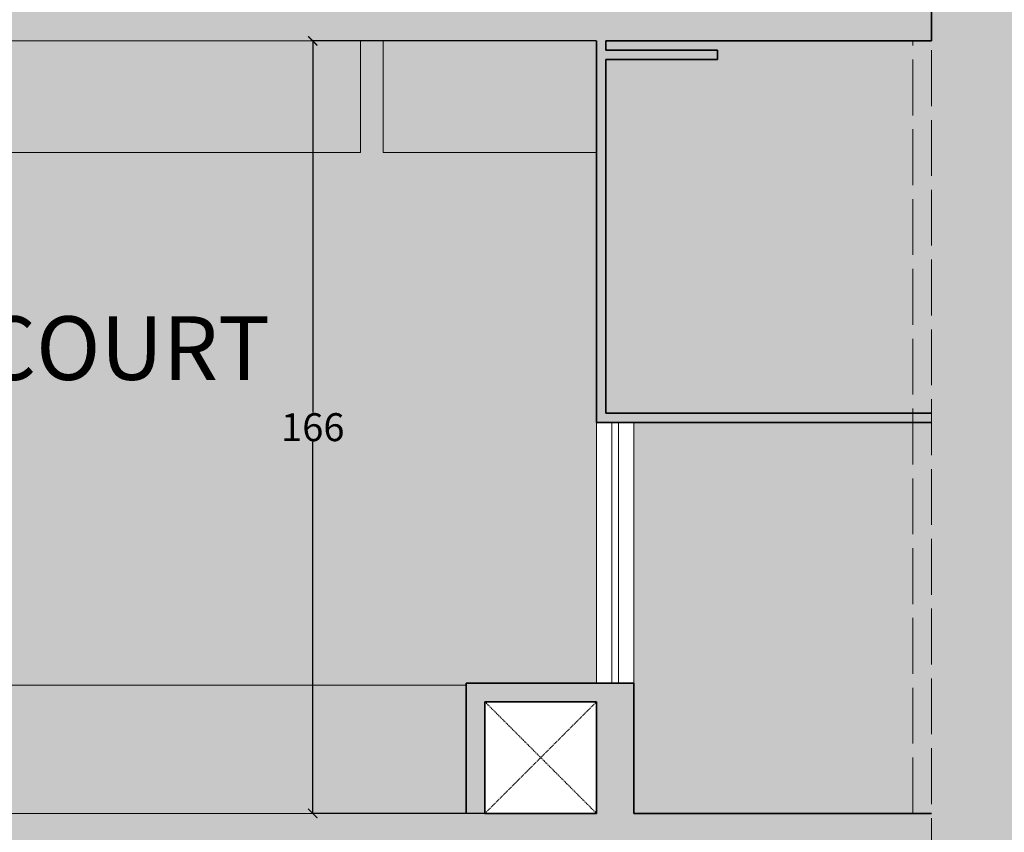
# Model space of a CAD drawing. Units: inches. Extents: x 1704 to 6393, y -157 to 1172.
# Tile 42 of 122: x 2081 to 2293, y 541 to 716. Entities that reach past the tile are written whole.
import ezdxf

# ---------------------------------------------------------------- set-up
doc = ezdxf.new("R2010")
doc.units = ezdxf.units.IN
doc.header["$MEASUREMENT"] = 0
doc.linetypes.add('ACAD_ISO02W100', pattern=[15, 12, -3])
doc.linetypes.add('HIDDEN', pattern=[0.375, 0.25, -0.125])
for name, color, linetype, lineweight in [('A-ANNO-DIMS', 7, 'Continuous', 13), ('A-AREA-IDEN', 7, 'Continuous', 18), ('A-FLOR-OPEN-HIDN', 8, 'HIDDEN', 13), ('A-WALL-OVHD', 8, 'ACAD_ISO02W100', 13), ('A-WALL-PATT', 7, 'Continuous', 13), ('GLASS PANEL FASADE', 4, 'Continuous', 18), ('L-HRDS', 8, 'Continuous', 18), ('WALLS', 7, 'Continuous', 35)]:
    doc.layers.add(name, color=color, linetype=linetype, lineweight=lineweight)
for name, color, linetype, lineweight, true_color in [('A-FLOR-PATT', 7, 'Continuous', 13, 0xf2f2f2), ('L-HRDS-PATT', 9, 'Continuous', 13, 0xc5c1ba), ('L-PLNT-PATT', 253, 'Continuous', 13, 0x9abc8f)]:
    doc.layers.add(name, color=color, linetype=linetype, lineweight=lineweight, true_color=true_color)
doc.styles.get("Standard").update_dxf_attribs({"font": 'arial.ttf'})
doc.dimstyles.get("Standard").update_dxf_attribs({"dimtxt": 6, "dimasz": 2, "dimexe": 0.18, "dimexo": 0.0625, "dimgap": 0.09, "dimtad": 0, "dimtih": 1, "dimtoh": 1, "dimdec": 1, "dimzin": 0, "dimdsep": 46, "dimlunit": 3, "dimtxsty": 'Standard', "dimblk": 'ARCHTICK', "dimcen": 0.09, "dimadec": 0, "dimazin": 0, "dimtfac": 1, "dimtdec": 1, "dimtofl": 0, "dimtmove": 0, "dimatfit": 3, "dimfxl": 1, "dimtolj": 1, "dimtzin": 0, "dimarcsym": 0})

# ---------------------------------------------------------------- blocks, each defined once
blk = doc.blocks.new('_ArchTick')
at = {"color": 0, "linetype": 'ByBlock', "const_width": 0.15}
blk.add_lwpolyline([(-0.5, -0.5), (0.5, 0.5)], dxfattribs=at)
blk = doc.blocks.new('*D93')
at = {"layer": 'A-ANNO-DIMS', "color": 0, "lineweight": -2, "transparency": 16777216}
for p, q in [((2605.29, 895.21), (1829.7, 895.21)), ((1829.88, 895.21), (1829.88, 495.87)), ((1829.88, 90.21), (1829.88, 489.56)), ((2605.29, 90.21), (1829.7, 90.21))]:
    blk.add_line(p, q, dxfattribs=at)
at = {"layer": 'Defpoints', "color": 0, "lineweight": -3, "transparency": 16777216}
for p in [(2605.35, 895.21), (1829.88, 90.21), (2605.35, 90.21)]:
    blk.add_point(p, dxfattribs=at)
at = {"layer": 'A-ANNO-DIMS', "color": 0, "lineweight": -2, "transparency": 16777216, "xscale": 2, "yscale": 2, "zscale": 2}
for p, rotation in [((1829.88, 895.21), 90), ((1829.88, 90.21), 270)]:
    blk.add_blockref('_ArchTick', p, dxfattribs=dict(at, rotation=rotation))
at = {"layer": 'A-ANNO-DIMS', "color": 0, "transparency": 16777216, "insert": (1829.88, 492.71), "char_height": 6, "attachment_point": 5}
blk.add_mtext('\\A1;805', dxfattribs=at)
blk = doc.blocks.new('*D96')
at = {"layer": 'A-ANNO-DIMS', "color": 0, "lineweight": -2, "transparency": 16777216}
for p, q in [((2205.29, 711.21), (2144.17, 711.21)), ((2144.35, 711.21), (2144.35, 631.37)), ((2144.35, 545.21), (2144.35, 625.06)), ((2205.29, 545.21), (2144.17, 545.21))]:
    blk.add_line(p, q, dxfattribs=at)
at = {"layer": 'Defpoints', "color": 0, "lineweight": -3, "transparency": 16777216}
for p in [(2144.35, 711.21), (2205.35, 711.21), (2205.35, 545.21)]:
    blk.add_point(p, dxfattribs=at)
at = {"layer": 'A-ANNO-DIMS', "color": 0, "lineweight": -2, "transparency": 16777216, "xscale": 2, "yscale": 2, "zscale": 2}
for p, rotation in [((2144.35, 711.21), 90), ((2144.35, 545.21), 270)]:
    blk.add_blockref('_ArchTick', p, dxfattribs=dict(at, rotation=rotation))
at = {"layer": 'A-ANNO-DIMS', "color": 0, "transparency": 16777216, "insert": (2144.35, 628.21), "char_height": 6, "attachment_point": 5}
blk.add_mtext('\\A1;166', dxfattribs=at)

msp = doc.modelspace()

# ---------------------------------------------------------------- hatches: boundary and pattern name
at = {"layer": 'A-FLOR-PATT', "transparency": 33554528}
h = msp.add_hatch(color=256, dxfattribs=at)
h.dxf.hatch_style = 1
h.paths.add_polyline_path([(2325.349, 863.213), (2325.349, 887.213), (2263.349, 887.213), (2167.349, 887.213), (2081.349, 887.213), (2081.349, 719.213), (2277.349, 719.213), (2277.349, 711.213), (2277.349, 372.213), (2349.349, 372.213), (2381.349, 372.213), (2381.349, 364.213), (2353.349, 364.213), (2353.349, 270.213), (2381.349, 270.213), (2381.349, 266.213), (2357.349, 266.213), (2357.349, 98.213), (2381.349, 98.213), (2385.181, 98.213), (2386.482, 98.213), (2424.215, 98.213), (2425.516, 98.213), (2429.349, 98.213), (2597.349, 98.213), (2597.349, 146.213), (2597.349, 218.213), (2597.349, 266.213), (2423.349, 266.213), (2423.349, 270.213), (2473.349, 270.213), (2473.349, 294.213), (2477.349, 294.213), (2477.349, 270.213), (2547.349, 270.213), (2547.349, 364.213), (2477.349, 364.213), (2477.349, 318.213), (2473.349, 318.213), (2473.349, 364.213), (2423.349, 364.213), (2423.349, 372.213), (2469.349, 372.213), (2469.349, 459.213), (2469.349, 538.213), (2350.349, 538.213), (2350.349, 565.713), (2358.349, 565.713), (2358.349, 545.213), (2420.349, 545.213), (2420.349, 610.213), (2358.349, 610.213), (2358.349, 589.713), (2350.349, 589.713), (2350.349, 615.213), (2425.349, 615.213), (2425.349, 607.213), (2425.349, 546.213), (2469.349, 546.213), (2514.349, 546.213), (2514.349, 607.213), (2449.349, 607.213), (2449.349, 615.213), (2451.738, 615.213), (2451.738, 659.213), (2427.738, 659.213), (2427.738, 665.213), (2367.738, 665.213), (2367.738, 667.213), (2367.738, 711.213), (2325.349, 711.213), (2325.349, 719.213), (2325.349, 755.213), (2325.349, 763.213)])
h.paths.add_polyline_path([(2233.858, 822.533, -0.187247), (2233.858, 809.14), (2231.697, 808.804, 0.0848928), (2233.131, 814.486), (2230.424, 814.486, -0.1042581), (2228.553, 808.313), (2217.751, 807.156, -0.2222222), (2217.751, 824.517), (2228.553, 823.359, -0.1042581), (2230.424, 817.186), (2233.131, 817.186, 0.0848928), (2231.697, 822.868)], flags=16)
h.paths.add_polyline_path([(2213.621, 833.197), (2213.621, 798.475), (2156.048, 798.475), (2156.048, 833.197)], flags=16)
h.paths.add_polyline_path([(2203.932, 848.099), (2205.089, 837.296, -0.2222222), (2187.728, 837.296), (2188.885, 848.099, -0.1042581), (2195.058, 849.969), (2195.058, 852.676, 0.0848928), (2189.377, 851.242), (2189.712, 853.404, -0.187247), (2203.105, 853.404), (2203.44, 851.242, 0.0848928), (2197.759, 852.676), (2197.759, 849.969, -0.1042581)], flags=16)
h.paths.add_polyline_path([(2181.941, 837.296, -0.2222222), (2164.58, 837.296), (2165.737, 848.099, -0.1042581), (2171.91, 849.969), (2171.91, 852.676, 0.0848928), (2166.229, 851.242), (2166.564, 853.404, -0.187247), (2179.957, 853.404), (2180.292, 851.242, 0.0848928), (2174.611, 852.676), (2174.611, 849.969, -0.1042581), (2180.784, 848.099)], flags=16)
h.paths.add_polyline_path([(2205.089, 794.376), (2203.932, 783.574, -0.1042581), (2197.759, 781.703), (2197.759, 778.996, 0.0848928), (2203.44, 780.43), (2203.105, 778.269, -0.187247), (2189.712, 778.269), (2189.377, 780.43, 0.0848928), (2195.058, 778.996), (2195.058, 781.703, -0.1042581), (2188.885, 783.574), (2187.728, 794.376, -0.2222222)], flags=16)
h.paths.add_polyline_path([(2181.941, 794.376), (2180.784, 783.574, -0.1042581), (2174.611, 781.703), (2174.611, 778.996, 0.0848928), (2180.292, 780.43), (2179.957, 778.269, -0.187247), (2166.564, 778.269), (2166.229, 780.43, 0.0848928), (2171.91, 778.996), (2171.91, 781.703, -0.1042581), (2165.737, 783.574), (2164.58, 794.376, -0.2222222)], flags=16)
h.paths.add_polyline_path([(2151.918, 807.156), (2141.116, 808.313, -0.1042581), (2139.245, 814.486), (2136.539, 814.486, 0.0848928), (2137.972, 808.804), (2135.811, 809.14, -0.187247), (2135.811, 822.533), (2137.972, 822.868, 0.0848928), (2136.539, 817.186), (2139.245, 817.186, -0.1042581), (2141.116, 823.359), (2151.918, 824.517, -0.2222222)], flags=16)
h.paths.add_polyline_path([(2357.868, 363.41), (2358.814, 363.41, 0.7537605)], flags=16)
h.paths.add_polyline_path([(2372.241, 363.117), (2372.248, 363.117), (2372.248, 363.343), (2371.302, 363.343), (2371.302, 363.139, -1.3603913)], flags=16)
h.paths.add_polyline_path([(2371.309, 272.716), (2371.302, 272.716), (2371.302, 272.49), (2372.248, 272.49), (2372.248, 272.693, -1.3603913)], flags=16)
h.paths.add_polyline_path([(2357.875, 272.716), (2357.868, 272.716), (2357.868, 272.49), (2358.814, 272.49), (2358.814, 272.693, -1.3603913)], flags=16)
h.paths.add_polyline_path([(2353.769, 363.074), (2376.347, 363.074), (2376.347, 272.759), (2353.769, 272.759)], flags=16)
h.paths.add_polyline_path([(2354.772, 362.07), (2375.344, 362.07), (2375.344, 273.762), (2354.772, 273.762)], flags=0)
h.paths.add_polyline_path([(2357.868, 363.343), (2358.814, 363.343), (2358.814, 363.117), (2357.868, 363.117)], flags=16)
h.paths.add_polyline_path([(2359.288, 359.184), (2359.288, 360.063), (2370.828, 360.063), (2370.828, 359.184), (2374.332, 359.184), (2374.332, 358.464), (2372.835, 358.464), (2372.835, 357.541), (2374.332, 357.541), (2374.332, 356.82), (2372.835, 356.82), (2372.835, 355.898), (2374.332, 355.898), (2374.332, 355.177), (2372.835, 355.177), (2372.835, 354.254), (2374.332, 354.254), (2374.332, 353.534), (2372.835, 353.534), (2372.835, 352.611), (2374.332, 352.611), (2374.332, 351.89), (2372.835, 351.89), (2372.835, 350.968), (2374.332, 350.968), (2374.332, 350.247), (2372.835, 350.247), (2372.835, 349.324), (2374.332, 349.324), (2374.332, 348.604), (2372.835, 348.604), (2372.835, 347.681), (2374.332, 347.681), (2374.332, 346.96), (2372.835, 346.96), (2372.835, 346.038), (2374.332, 346.038), (2374.332, 345.317), (2372.835, 345.317), (2372.835, 344.395), (2374.332, 344.395), (2374.332, 343.674), (2372.835, 343.674), (2372.835, 342.751), (2374.332, 342.751), (2374.332, 342.03), (2372.835, 342.03), (2372.835, 341.108), (2374.332, 341.108), (2374.332, 340.387), (2372.835, 340.387), (2372.835, 339.465), (2374.332, 339.465), (2374.332, 338.744), (2372.835, 338.744), (2372.835, 337.821), (2374.332, 337.821), (2374.332, 337.1), (2372.835, 337.1), (2372.835, 336.178), (2374.332, 336.178), (2374.332, 335.457), (2372.835, 335.457), (2372.835, 334.535), (2374.332, 334.535), (2374.332, 333.814), (2372.835, 333.814), (2372.835, 332.891), (2374.332, 332.891), (2374.332, 332.171), (2372.835, 332.171), (2372.835, 331.248), (2374.332, 331.248), (2374.332, 330.527), (2372.835, 330.527), (2372.835, 329.605), (2374.332, 329.605), (2374.332, 328.884), (2372.835, 328.884), (2372.835, 327.961), (2374.332, 327.961), (2374.332, 327.241), (2372.835, 327.241), (2372.835, 326.318), (2374.332, 326.318), (2374.332, 325.597), (2372.835, 325.597), (2372.835, 324.675), (2374.332, 324.675), (2374.332, 323.954), (2372.835, 323.954), (2372.835, 323.031), (2374.332, 323.031), (2374.332, 322.311), (2372.835, 322.311), (2372.835, 321.388), (2374.332, 321.388), (2374.332, 320.667), (2372.835, 320.667), (2372.835, 319.745), (2374.332, 319.745), (2374.332, 319.024), (2372.835, 319.024), (2372.835, 318.102), (2374.332, 318.102), (2374.332, 317.381), (2372.835, 317.381), (2372.835, 316.458), (2374.332, 316.458), (2374.332, 315.737), (2372.835, 315.737), (2372.835, 314.815), (2374.332, 314.815), (2374.332, 314.094), (2372.835, 314.094), (2372.835, 313.172), (2374.332, 313.172), (2374.332, 312.451), (2372.835, 312.451), (2372.835, 311.528), (2374.332, 311.528), (2374.332, 310.807), (2372.835, 310.807), (2372.835, 309.885), (2374.332, 309.885), (2374.332, 309.164), (2372.835, 309.164), (2372.835, 308.242), (2374.332, 308.242), (2374.332, 307.521), (2372.835, 307.521), (2372.835, 306.598), (2374.332, 306.598), (2374.332, 305.878), (2372.835, 305.878), (2372.835, 304.955), (2374.332, 304.955), (2374.332, 304.234), (2372.835, 304.234), (2372.835, 303.312), (2374.332, 303.312), (2374.332, 302.591), (2372.835, 302.591), (2372.835, 301.668), (2374.332, 301.668), (2374.332, 300.948), (2372.835, 300.948), (2372.835, 300.025), (2374.332, 300.025), (2374.332, 299.304), (2372.835, 299.304), (2372.835, 298.382), (2374.332, 298.382), (2374.332, 297.661), (2372.835, 297.661), (2372.835, 296.738), (2374.332, 296.738), (2374.332, 296.018), (2372.835, 296.018), (2372.835, 295.095), (2374.332, 295.095), (2374.332, 294.374), (2372.835, 294.374), (2372.835, 293.452), (2374.332, 293.452), (2374.332, 292.731), (2372.835, 292.731), (2372.835, 291.809), (2374.332, 291.809), (2374.332, 291.088), (2372.835, 291.088), (2372.835, 290.165), (2374.332, 290.165), (2374.332, 289.444), (2372.835, 289.444), (2372.835, 288.522), (2374.332, 288.522), (2374.332, 287.801), (2372.835, 287.801), (2372.835, 286.879), (2374.332, 286.879), (2374.332, 286.158), (2372.835, 286.158), (2372.835, 285.235), (2374.332, 285.235), (2374.332, 284.514), (2372.835, 284.514), (2372.835, 283.592), (2374.332, 283.592), (2374.332, 282.871), (2372.835, 282.871), (2372.835, 281.949), (2374.332, 281.949), (2374.332, 281.228), (2372.835, 281.228), (2372.835, 280.305), (2374.332, 280.305), (2374.332, 279.585), (2372.835, 279.585), (2372.835, 278.662), (2374.332, 278.662), (2374.332, 277.941), (2372.835, 277.941), (2372.835, 277.019), (2374.332, 277.019), (2374.332, 276.298), (2370.828, 276.298), (2370.828, 275.769), (2359.288, 275.769), (2359.288, 276.298), (2355.784, 276.298), (2355.784, 277.019), (2357.281, 277.019), (2357.281, 277.941), (2355.784, 277.941), (2355.784, 278.662), (2357.281, 278.662), (2357.281, 279.585), (2355.784, 279.585), (2355.784, 280.305), (2357.281, 280.305), (2357.281, 281.228), (2355.784, 281.228), (2355.784, 281.949), (2357.281, 281.949), (2357.281, 282.871), (2355.784, 282.871), (2355.784, 283.592), (2357.281, 283.592), (2357.281, 284.514), (2355.784, 284.514), (2355.784, 285.235), (2357.281, 285.235), (2357.281, 286.158), (2355.784, 286.158), (2355.784, 286.879), (2357.281, 286.879), (2357.281, 287.801), (2355.784, 287.801), (2355.784, 288.522), (2357.281, 288.522), (2357.281, 289.444), (2355.784, 289.444), (2355.784, 290.165), (2357.281, 290.165), (2357.281, 291.088), (2355.784, 291.088), (2355.784, 291.809), (2357.281, 291.809), (2357.281, 292.731), (2355.784, 292.731), (2355.784, 293.452), (2357.281, 293.452), (2357.281, 294.374), (2355.784, 294.374), (2355.784, 295.095), (2357.281, 295.095), (2357.281, 296.018), (2355.784, 296.018), (2355.784, 296.738), (2357.281, 296.738), (2357.281, 297.661), (2355.784, 297.661), (2355.784, 298.382), (2357.281, 298.382), (2357.281, 299.304), (2355.784, 299.304), (2355.784, 300.025), (2357.281, 300.025), (2357.281, 300.948), (2355.784, 300.948), (2355.784, 301.668), (2357.281, 301.668), (2357.281, 302.591), (2355.784, 302.591), (2355.784, 303.312), (2357.281, 303.312), (2357.281, 304.234), (2355.784, 304.234), (2355.784, 304.955), (2357.281, 304.955), (2357.281, 305.878), (2355.784, 305.878), (2355.784, 306.598), (2357.281, 306.598), (2357.281, 307.521), (2355.784, 307.521), (2355.784, 308.242), (2357.281, 308.242), (2357.281, 309.164), (2355.784, 309.164), (2355.784, 309.885), (2357.281, 309.885), (2357.281, 310.807), (2355.784, 310.807), (2355.784, 311.528), (2357.281, 311.528), (2357.281, 312.451), (2355.784, 312.451), (2355.784, 313.172), (2357.281, 313.172), (2357.281, 314.094), (2355.784, 314.094), (2355.784, 314.815), (2357.281, 314.815), (2357.281, 315.737), (2355.784, 315.737), (2355.784, 316.458), (2357.281, 316.458), (2357.281, 317.381), (2355.784, 317.381), (2355.784, 318.102), (2357.281, 318.102), (2357.281, 319.024), (2355.784, 319.024), (2355.784, 319.745), (2357.281, 319.745), (2357.281, 320.667), (2355.784, 320.667), (2355.784, 321.388), (2357.281, 321.388), (2357.281, 322.311), (2355.784, 322.311), (2355.784, 323.031), (2357.281, 323.031), (2357.281, 323.954), (2355.784, 323.954), (2355.784, 324.675), (2357.281, 324.675), (2357.281, 325.597), (2355.784, 325.597), (2355.784, 326.318), (2357.281, 326.318), (2357.281, 327.241), (2355.784, 327.241), (2355.784, 327.961), (2357.281, 327.961), (2357.281, 328.884), (2355.784, 328.884), (2355.784, 329.605), (2357.281, 329.605), (2357.281, 330.527), (2355.784, 330.527), (2355.784, 331.248), (2357.281, 331.248), (2357.281, 332.171), (2355.784, 332.171), (2355.784, 332.891), (2357.281, 332.891), (2357.281, 333.814), (2355.784, 333.814), (2355.784, 334.535), (2357.281, 334.535), (2357.281, 335.457), (2355.784, 335.457), (2355.784, 336.178), (2357.281, 336.178), (2357.281, 337.1), (2355.784, 337.1), (2355.784, 337.821), (2357.281, 337.821), (2357.281, 338.744), (2355.784, 338.744), (2355.784, 339.465), (2357.281, 339.465), (2357.281, 340.387), (2355.784, 340.387), (2355.784, 341.108), (2357.281, 341.108), (2357.281, 342.03), (2355.784, 342.03), (2355.784, 342.751), (2357.281, 342.751), (2357.281, 343.674), (2355.784, 343.674), (2355.784, 344.395), (2357.281, 344.395), (2357.281, 345.317), (2355.784, 345.317), (2355.784, 346.038), (2357.281, 346.038), (2357.281, 346.96), (2355.784, 346.96), (2355.784, 347.681), (2357.281, 347.681), (2357.281, 348.604), (2355.784, 348.604), (2355.784, 349.324), (2357.281, 349.324), (2357.281, 350.247), (2355.784, 350.247), (2355.784, 350.968), (2357.281, 350.968), (2357.281, 351.89), (2355.784, 351.89), (2355.784, 352.611), (2357.281, 352.611), (2357.281, 353.534), (2355.784, 353.534), (2355.784, 354.254), (2357.281, 354.254), (2357.281, 355.177), (2355.784, 355.177), (2355.784, 355.898), (2357.281, 355.898), (2357.281, 356.82), (2355.784, 356.82), (2355.784, 357.541), (2357.281, 357.541), (2357.281, 358.464), (2355.784, 358.464), (2355.784, 359.184)], flags=0)
h = msp.add_hatch(color=256, dxfattribs=at)
h.dxf.hatch_style = 1
h.paths.add_polyline_path([(2273.349, 538.213), (2081.349, 538.213), (2081.349, 372.213), (2273.349, 372.213)])
h.paths.add_polyline_path([(2189.542, 505.951), (2184.316, 505.951), (2184.316, 505.591), (2169.442, 505.591), (2169.442, 505.951), (2164.216, 505.951, -0.4142136), (2163.814, 506.353), (2163.814, 526.093, -0.4142136), (2164.216, 526.495), (2189.542, 526.495, -0.4142136), (2189.944, 526.093), (2189.944, 506.353, -0.4142136)], flags=16)
h.paths.add_polyline_path([(2200.535, 511.491), (2200.535, 526.191), (2217.621, 526.191), (2217.621, 511.491), (2214.605, 511.491, -0.3946213), (2214.203, 511.116), (2203.952, 511.116, -0.3946213), (2203.551, 511.491)], flags=16)
h.paths.add_polyline_path([(2200.736, 511.692), (2200.736, 525.99), (2203.55, 525.99), (2203.55, 523.838, 0.1045605), (2214.605, 523.838), (2214.605, 525.99), (2217.42, 525.99), (2217.42, 511.692), (2214.605, 511.692), (2214.605, 523.838, -0.1045605), (2203.55, 523.838), (2203.55, 511.692)], flags=0)
h.paths.add_polyline_path([(2203.952, 511.317, -0.4142136), (2203.751, 511.518), (2203.751, 523.591, 0.099912), (2214.404, 523.591), (2214.404, 511.518, -0.4142136), (2214.203, 511.317)], flags=0)
h.paths.add_polyline_path([(2184.084, 516.015, -0.0686795), (2169.674, 516.015), (2169.674, 522.073), (2184.084, 522.073)], flags=0)
h.paths.add_polyline_path([(2183.325, 518.606, -0.0772766), (2170.433, 518.606), (2170.433, 521.123, -0.0235462), (2183.325, 521.123)], flags=0)
h.paths.add_polyline_path([(2135.029, 507.225, -0.1405189), (2135.191, 507.834, -0.0513838), (2135.029, 507.797)], flags=16)
h.paths.add_polyline_path([(2146.318, 498.997, -0.0311848), (2144.279, 499.202, -0.1719602), (2141.865, 499.263, -0.2234326), (2139.482, 499.263, -0.1719602), (2137.068, 499.202, -0.0311848), (2135.029, 498.997, -0.066975), (2135.029, 505.313, -0.0276914), (2136.841, 505.144), (2136.841, 506.777), (2136.576, 506.777), (2136.576, 507.371, 0.039911), (2145.741, 507.448, 0.2546956), (2146.318, 507.225), (2146.318, 507.269, 0.1305786), (2146.156, 507.834, -0.0704067), (2145.953, 507.935, -0.011584), (2145.714, 508.002, -0.2546956), (2145.137, 507.779, -0.2546956), (2145.361, 508.355, -0.0259693), (2145.107, 516.407, -0.0070422), (2144.025, 516.297, -0.1828112), (2142.939, 516.218, -0.2042746), (2142.015, 516.175, -0.1805419), (2139.348, 516.174, -0.0000184), (2139.345, 516.174, -0.2035615), (2138.425, 516.217, -0.0000237), (2138.421, 516.217, -0.1818152), (2137.34, 516.296, -0.0071635), (2136.24, 516.407, 0.007166), (2136.162, 518.63, 0.314303), (2135.854, 518.974, -0.1253469), (2135.537, 518.935, -0.2546956), (2135.76, 519.512, -0.0162662), (2135.67, 519.849, -0.296972), (2135.535, 520.8, -0.227702), (2135.464, 521.698, 0.1283977), (2132.757, 521.718), (2132.757, 525.785, -0.4142136), (2133.331, 526.359), (2148.015, 526.359, -0.4142136), (2148.589, 525.785), (2148.589, 521.718, -0.0118936), (2148.835, 521.65, -0.2546956), (2149.412, 521.873, -0.2546956), (2149.188, 521.296, -0.0417628), (2149.188, 508.355, -0.2546956), (2149.412, 507.779, -0.2546956), (2148.835, 508.002, -0.011584), (2148.596, 507.935, -0.2124435), (2147.949, 507.813, -0.2363999), (2147.423, 507.772, -0.3143526), (2147.126, 507.772, -0.2363999), (2146.6, 507.813, -0.0879275), (2146.318, 507.797), (2146.318, 507.225, -0.2546956), (2145.741, 507.448, -0.0042329), (2144.771, 507.371), (2144.771, 506.777), (2144.506, 506.777), (2144.506, 505.144, -0.0276914), (2146.318, 505.313, -0.066975)], flags=16)
h.paths.add_polyline_path([(2141.865, 505.047, 0.2234326), (2139.482, 505.047, 0.1738145), (2137.043, 505.1), (2137.043, 506.317), (2137.335, 506.317), (2137.335, 505.184, -0.1522072), (2139.482, 505.047, -0.2234326), (2141.865, 505.047, -0.1522072), (2144.011, 505.184), (2144.011, 506.317), (2144.304, 506.317), (2144.304, 505.1, 0.1738145)], flags=0)
h.paths.add_polyline_path([(2145.233, 522.986, 0.0079197), (2144.017, 523.111, 0.1826165), (2142.931, 523.19, 0.2042746), (2142.008, 523.233, 0.1806536), (2139.339, 523.233, 0.2042746), (2138.415, 523.19, 0.1826165), (2137.33, 523.111, 0.0079197), (2136.114, 522.986, 0.1967082), (2135.679, 523.212, 0.047677), (2135.755, 524.004), (2134.638, 521.852), (2134.376, 524.691, -0.2583282), (2135.029, 526.359, -0.0890464), (2135.632, 525.01, -0.1830277), (2145.715, 525.01, -0.0890464), (2146.318, 526.359, -0.2583282), (2146.971, 524.691), (2146.709, 521.852), (2145.592, 524.004, 0.047677), (2145.668, 523.212, 0.1967082)], flags=0)
h.paths.add_polyline_path([(2144.419, 519.027, -0.0368796), (2136.927, 519.027, -0.0368796)], flags=0)
h.paths.add_polyline_path([(2273.349, 629.213), (2213.349, 629.213), (2213.349, 573.213), (2213.349, 545.213), (2273.349, 545.213)])
h.paths.add_polyline_path([(2273.349, 711.213), (2207.349, 711.213), (2207.349, 709.213), (2231.349, 709.213), (2231.349, 707.213), (2207.349, 707.213), (2207.349, 631.213), (2273.349, 631.213)])
h.paths.add_polyline_path([(2273.349, 364.213), (2081.349, 364.213), (2081.349, 202.213), (2225.349, 202.213), (2229.181, 202.213), (2230.482, 202.213), (2268.215, 202.213), (2269.516, 202.213), (2273.349, 202.213)])
h.paths.add_polyline_path([(2203.551, 339.558, 0.3946213), (2203.952, 339.183), (2214.203, 339.183), (2214.203, 339.384), (2203.751, 339.384), (2203.751, 339.558)], flags=16)
h.paths.add_polyline_path([(2203.55, 351.7), (2203.55, 339.759), (2200.535, 339.759), (2200.535, 354.258), (2217.621, 354.258), (2217.621, 339.558), (2214.404, 339.558), (2214.404, 351.659, -0.101837)], flags=16)
h.paths.add_polyline_path([(2214.404, 354.057), (2214.605, 354.057), (2214.605, 354.258), (2214.404, 354.258)], flags=16)
h.paths.add_polyline_path([(2189.542, 334.018), (2184.316, 334.018), (2184.316, 333.658), (2169.442, 333.658), (2169.442, 334.018), (2164.216, 334.018, -0.4142136), (2163.814, 334.42), (2163.814, 354.161, -0.4142136), (2164.216, 354.563), (2189.542, 354.563, -0.4142136), (2189.944, 354.161), (2189.944, 334.42, -0.4142136)], flags=16)
h.paths.add_polyline_path([(2184.084, 344.083, -0.0686795), (2169.674, 344.083), (2169.674, 349.85), (2165.7, 350.14), (2188.058, 350.14), (2184.084, 349.85)], flags=0)
h.paths.add_polyline_path([(2183.325, 346.673, -0.0772766), (2170.433, 346.673), (2170.433, 349.19, -0.0235462), (2183.325, 349.19)], flags=0)
h.paths.add_polyline_path([(2134.638, 349.919), (2134.376, 352.758, -0.2583282), (2135.029, 354.426), (2133.331, 354.426, 0.4142136), (2132.757, 353.852), (2132.757, 349.785, -0.0886664)], flags=16)
h.paths.add_polyline_path([(2136.114, 351.053, -0.0079197), (2137.33, 351.178, -0.1826165), (2138.415, 351.257, -0.2042746), (2139.339, 351.3, -0.1806536), (2142.008, 351.3, -0.2042746), (2142.931, 351.257, -0.1826165), (2144.017, 351.178, -0.0079197), (2145.233, 351.053, -0.1967082), (2145.668, 351.279, -0.047677), (2145.592, 352.071, 0.1133241), (2135.755, 352.071, -0.047677), (2135.679, 351.279, -0.1967082)], flags=16)
h.paths.add_polyline_path([(2145.184, 346.697, 0.0331414), (2145.361, 336.423, 0.2546956), (2145.137, 335.846, 0.3030408), (2145.781, 336.164, 0.2903634), (2146.6, 335.88, 0.2363999), (2147.126, 335.839, -0.280712), (2147.275, 336.69, -0.280712), (2147.423, 335.839, 0.2363999), (2147.949, 335.88, 0.2903634), (2148.768, 336.164, 0.3030408), (2149.412, 335.846, 0.2546956), (2149.188, 336.423, 0.0417628), (2149.188, 349.363, 0.2546956), (2149.412, 349.94, 0.2546956), (2148.835, 349.717, 0.1405058), (2145.883, 349.765, -0.227702), (2145.812, 348.867, -0.296972), (2145.677, 347.916, -0.0162662), (2145.586, 347.579, -0.2546956), (2145.81, 347.002, -0.1253469), (2145.493, 347.041, 0.314303)], flags=16)
h.paths.add_polyline_path([(2135.029, 335.292, -0.1405189), (2135.191, 335.901, -0.1399435), (2134.747, 335.88, -0.2363999), (2134.22, 335.839, -0.3143526), (2133.924, 335.839, -0.280712), (2134.072, 336.69, -0.280712), (2134.22, 335.839, 0.2363999), (2134.747, 335.88, 0.2903634), (2135.566, 336.164, 0.3030408), (2136.209, 335.846, 0.2546956), (2135.985, 336.423, 0.0331414), (2136.162, 346.697, 0.314303), (2135.854, 347.041, -0.1253469), (2135.537, 347.002, -0.2546956), (2135.76, 347.579, -0.0162662), (2135.67, 347.916, -0.296972), (2135.535, 348.867, -0.2999866), (2135.599, 350.01, -0.0330719), (2135.76, 350.7, -0.3502076), (2135.604, 351.492), (2134.638, 349.919), (2135.604, 351.492, 0.3502076), (2135.76, 350.7, 0.0330719), (2135.599, 350.01, 0.2999866), (2135.535, 348.867, 0.296972), (2135.67, 347.916, 0.0279375), (2135.971, 347.698, 0.3576436), (2135.537, 347.002, 0.1253469), (2135.854, 347.041, -0.3555912), (2136.165, 346.637, -0.0329482), (2135.985, 336.423, -0.2546956), (2136.209, 335.846, -0.2546956), (2135.632, 336.069, -0.011584), (2135.393, 336.003, -0.1222327), (2135.029, 335.864)], flags=16)
h.paths.add_polyline_path([(2136.841, 335.42), (2136.783, 335.423), (2136.783, 334.844), (2136.841, 334.471)], flags=16)
h.paths.add_polyline_path([(2146.318, 327.064, -0.0311848), (2144.279, 327.269, -0.1719602), (2141.865, 327.33, -0.2234326), (2139.482, 327.33, -0.1719602), (2137.068, 327.269, -0.0311848), (2135.029, 327.064, -0.066975), (2135.029, 333.38, -0.0311848), (2137.068, 333.175, -0.1719602), (2139.482, 333.114, -0.2234326), (2141.865, 333.114, -0.1522072), (2144.011, 333.251), (2144.011, 334.384), (2144.304, 335.406, 0.0020345), (2144.771, 335.438), (2144.771, 334.844), (2144.506, 333.211, -0.0276914), (2146.318, 333.38, -0.066975)], flags=16)
h.paths.add_polyline_path([(2137.129, 334.384), (2137.335, 334.384), (2137.335, 333.251), (2137.129, 333.195)], flags=16)
h.paths.add_polyline_path([(2144.419, 347.094, -0.0368796), (2136.927, 347.094, -0.0368796)], flags=16)
h = msp.add_hatch(color=256, dxfattribs=at)
h.dxf.hatch_style = 1
h.paths.add_polyline_path([(2349.349, 372.213), (2277.349, 372.213), (2277.349, 364.213), (2349.349, 364.213)])
h.paths.add_polyline_path([(2277.349, 372.213), (2273.349, 372.213), (2273.349, 364.213), (2277.349, 364.213)])
h.paths.add_polyline_path([(2277.349, 364.213), (2273.349, 364.213), (2273.349, 202.213), (2277.349, 202.213)])
h.paths.add_polyline_path([(2277.349, 538.213), (2273.349, 538.213), (2273.349, 372.213), (2277.349, 372.213)])
h.paths.add_polyline_path([(2277.349, 629.213), (2273.349, 629.213), (2273.349, 545.213), (2277.349, 545.213)])
h.paths.add_polyline_path([(2277.349, 711.213), (2273.349, 711.213), (2273.349, 631.213), (2277.349, 631.213)])
h.paths.add_polyline_path([(2277.349, 631.213), (2273.349, 631.213), (2273.349, 629.213), (2277.349, 629.213)])
at = {"layer": 'A-WALL-PATT', "transparency": 33554643}
h = msp.add_hatch(color=256, dxfattribs=at)
h.dxf.hatch_style = 1
h.paths.add_polyline_path([(2167.349, 895.213), (2073.349, 895.213), (2073.349, 887.213), (2081.349, 887.213), (2167.349, 887.213)])
h.paths.add_polyline_path([(2465.349, 895.213), (2273.349, 895.213), (2273.349, 903.213), (2263.349, 903.213), (2263.349, 895.213), (2263.349, 887.213), (2325.349, 887.213), (2325.349, 863.213), (2333.349, 863.213), (2333.349, 887.213), (2465.349, 887.213)])
h.paths.add_polyline_path([(2533.349, 895.213), (2513.349, 895.213), (2513.349, 887.213), (2513.349, 861.213), (2517.349, 861.213), (2517.349, 887.213), (2533.349, 887.213)])
h.paths.add_polyline_path([(2605.349, 895.213), (2581.349, 895.213), (2581.349, 887.213), (2597.349, 887.213), (2597.349, 854.213), (2605.349, 854.213)])
h.paths.add_polyline_path([(2605.349, 752.213), (2629.349, 752.213), (2629.349, 716.213), (2605.349, 716.213), (2605.349, 712.213), (2719.349, 712.213), (2719.349, 716.213), (2631.349, 716.213), (2631.349, 754.213), (2605.349, 754.213), (2605.349, 794.213), (2597.349, 794.213), (2597.349, 787.213), (2517.349, 787.213), (2517.349, 813.213), (2513.349, 813.213), (2513.349, 783.213), (2517.349, 783.213), (2597.349, 783.213), (2597.349, 719.213), (2517.349, 719.213), (2517.349, 753.213), (2513.349, 753.213), (2513.349, 719.213), (2365.349, 719.213), (2365.349, 763.213), (2325.349, 763.213), (2325.349, 755.213), (2357.349, 755.213), (2357.349, 719.213), (2325.349, 719.213), (2325.349, 711.213), (2547.349, 711.213), (2547.349, 615.213), (2449.349, 615.213), (2449.349, 607.213), (2514.349, 607.213), (2514.349, 546.213), (2439.349, 546.213), (2425.349, 546.213), (2425.349, 607.213), (2425.349, 615.213), (2350.349, 615.213), (2350.349, 589.713), (2358.349, 589.713), (2358.349, 610.213), (2420.349, 610.213), (2420.349, 545.213), (2358.349, 545.213), (2358.349, 565.713), (2350.349, 565.713), (2350.349, 538.213), (2469.349, 538.213), (2469.349, 459.213), (2469.349, 372.213), (2423.349, 372.213), (2423.349, 364.213), (2473.349, 364.213), (2473.349, 318.213), (2477.349, 318.213), (2477.349, 364.213), (2547.349, 364.213), (2547.349, 352.213), (2549.349, 352.213), (2549.349, 364.213), (2597.349, 364.213), (2597.349, 328.213), (2549.349, 328.213), (2547.349, 328.213), (2547.349, 326.213), (2549.349, 326.213), (2597.349, 326.213), (2605.349, 326.213), (2605.349, 377.057), (2597.349, 377.057), (2597.349, 372.213), (2477.349, 372.213), (2477.349, 451.213), (2597.349, 451.213), (2605.349, 451.213), (2605.349, 459.213), (2597.349, 459.213), (2477.349, 459.213), (2477.349, 538.213), (2597.349, 538.213), (2597.349, 495.213), (2605.349, 495.213), (2605.349, 512.213), (2631.349, 512.213), (2631.349, 568.213), (2605.349, 568.213), (2605.349, 577.213), (2597.349, 577.213), (2597.349, 542.213), (2518.349, 542.213), (2518.349, 607.213), (2532.349, 607.213), (2605.349, 607.213), (2605.349, 615.213), (2597.349, 615.213), (2551.349, 615.213), (2551.349, 711.213), (2597.349, 711.213), (2597.349, 645.213), (2605.349, 645.213), (2605.349, 712.213), (2605.349, 716.213)])
h.paths.add_polyline_path([(2605.349, 566.213), (2629.349, 566.213), (2629.349, 514.213), (2605.349, 514.213)], flags=16)
h.paths.add_polyline_path([(2381.349, 372.213), (2349.349, 372.213), (2349.349, 202.213), (2337.349, 202.213), (2337.349, 194.213), (2349.349, 194.213), (2349.349, 90.213), (2349.349, 72.213), (2357.349, 72.213), (2357.349, 90.213), (2381.349, 90.213), (2381.349, 98.213), (2357.349, 98.213), (2357.349, 266.213), (2381.349, 266.213), (2381.349, 270.213), (2353.349, 270.213), (2353.349, 364.213), (2381.349, 364.213)])
h.paths.add_polyline_path([(2605.349, 302.213), (2597.349, 302.213), (2597.349, 270.213), (2477.349, 270.213), (2477.349, 294.213), (2473.349, 294.213), (2473.349, 270.213), (2423.349, 270.213), (2423.349, 266.213), (2597.349, 266.213), (2597.349, 218.213), (2605.349, 218.213)])
h.paths.add_polyline_path([(2605.349, 146.213), (2597.349, 146.213), (2597.349, 98.213), (2429.349, 98.213), (2429.349, 90.213), (2597.349, 90.213), (2597.349, 72.213), (2605.349, 72.213), (2605.349, 90.213)])
h.paths.add_polyline_path([(2225.349, 202.213), (2049.349, 202.213), (2049.349, 194.213), (2225.349, 194.213)])
h.paths.add_polyline_path([(2289.349, 202.213), (2277.349, 202.213), (2273.349, 202.213), (2269.516, 202.213), (2269.516, 194.213), (2273.349, 194.213), (2277.349, 194.213), (2289.349, 194.213)])
h.paths.add_polyline_path([(2273.349, 372.213), (2029.19, 372.213), (2029.19, 364.213), (2273.349, 364.213)])
h.paths.add_polyline_path([(2277.349, 545.213), (2213.349, 545.213), (2213.349, 573.213), (2205.349, 573.213), (2177.349, 573.213), (2177.349, 545.213), (2073.349, 545.213), (2073.349, 538.213), (2081.349, 538.213), (2277.349, 538.213)])
h.paths.add_polyline_path([(2181.349, 545.213), (2181.349, 569.213), (2205.349, 569.213), (2205.349, 545.213)], flags=16)
h.paths.add_polyline_path([(2277.349, 719.213), (2081.349, 719.213), (2073.349, 719.213), (2073.349, 711.213), (2154.575, 711.213), (2205.349, 711.213), (2205.349, 687.213), (2205.349, 629.213), (2213.349, 629.213), (2273.349, 629.213), (2273.349, 631.213), (2207.349, 631.213), (2207.349, 707.213), (2231.349, 707.213), (2231.349, 709.213), (2207.349, 709.213), (2207.349, 711.213), (2277.349, 711.213)])
at = {"layer": 'L-HRDS-PATT', "transparency": 33554643}
h = msp.add_hatch(color=256, dxfattribs=at)
h.dxf.hatch_style = 1
h.paths.add_polyline_path([(2154.575, 711.213), (1958.127, 711.213), (1958.127, 687.213), (2154.575, 687.213)])
h.paths.add_polyline_path([(2205.349, 711.213), (2159.484, 711.213), (2159.484, 687.213), (2205.349, 687.213)])
h.paths.add_polyline_path([(2177.349, 572.777), (2008.58, 572.777), (2008.58, 545.213), (2177.349, 545.213)])
at = {"layer": 'L-PLNT-PATT', "transparency": 33554643}
h = msp.add_hatch(color=256, dxfattribs=at)
h.dxf.hatch_style = 1
h.paths.add_polyline_path([(2205.349, 687.213), (2159.484, 687.213), (2159.484, 711.213), (2154.575, 711.213), (2154.575, 687.213), (1958.127, 687.213), (1958.127, 711.213), (1898.349, 711.213), (1898.349, 545.213), (2008.58, 545.213), (2008.58, 572.777), (2177.349, 572.777), (2177.349, 573.213), (2205.349, 573.213), (2205.349, 629.213)])

# ---------------------------------------------------------------- linework, layer by layer
at = {"layer": 'A-FLOR-OPEN-HIDN'}
for p, q in [((2181.349, 545.213), (2205.349, 569.213)), ((2181.349, 569.213), (2205.349, 545.213))]:
    msp.add_line(p, q, dxfattribs=at)
at = {"layer": 'A-WALL-OVHD'}
for p, q in [((2273.349, 545.213), (2273.349, 711.213)), ((2277.349, 202.213), (2277.349, 711.213))]:
    msp.add_line(p, q, dxfattribs=at)
at = {"layer": 'GLASS PANEL FASADE'}
for p, q in [((2208.649, 573.213), (2208.649, 629.213)), ((2210.049, 573.213), (2210.049, 629.213))]:
    msp.add_line(p, q, dxfattribs=at)
msp.add_lwpolyline([(2213.349, 573.213), (2205.349, 573.213), (2205.349, 629.213), (2213.349, 629.213)], close=True, dxfattribs=at)
at = {"layer": 'L-HRDS'}
for p, q in [((2205.349, 711.213), (1898.349, 711.213)), ((2177.349, 545.213), (2073.349, 545.213))]:
    msp.add_line(p, q, dxfattribs=at)
for points in [[(2154.575, 711.213), (1958.127, 711.213), (1958.127, 687.213), (2154.575, 687.213)], [(2205.349, 711.213), (2159.484, 711.213), (2159.484, 687.213), (2205.349, 687.213)], [(2177.349, 545.213), (2008.58, 545.213), (2008.58, 572.777), (2177.349, 572.777)]]:
    msp.add_lwpolyline(points, close=True, dxfattribs=at)
at = {"layer": 'WALLS'}
for p, q in [((2277.349, 719.213), (2277.349, 711.213)), ((2205.349, 629.213), (2205.349, 711.213)), ((2207.349, 709.213), (2207.349, 711.213)), ((2277.349, 711.213), (2207.349, 711.213)), ((2231.349, 709.213), (2207.349, 709.213)), ((2231.349, 707.213), (2231.349, 709.213)), ((2207.349, 631.213), (2207.349, 707.213)), ((2207.349, 707.213), (2231.349, 707.213)), ((2277.349, 631.213), (2207.349, 631.213)), ((2277.349, 629.213), (2205.349, 629.213)), ((2177.349, 573.213), (2177.349, 545.213)), ((2177.349, 573.213), (2205.349, 573.213)), ((2205.349, 573.213), (2213.349, 573.213)), ((2213.349, 545.213), (2213.349, 573.213)), ((2181.349, 569.213), (2205.349, 569.213)), ((2181.349, 569.213), (2181.349, 545.213)), ((2205.349, 545.213), (2205.349, 569.213)), ((2205.349, 545.213), (2181.349, 545.213)), ((2277.349, 545.213), (2213.349, 545.213))]:
    msp.add_line(p, q, dxfattribs=at)

# ---------------------------------------------------------------- texts
at = {"layer": 'A-AREA-IDEN'}
msp.add_text('LANDSCAPE COURT', height=13.6672, dxfattribs=at).set_placement((1963.906, 638.365))

# ---------------------------------------------------------------- dimensions: what is measured, and where the dimension line sits
at = {"layer": 'A-ANNO-DIMS'}
for base, p1, p2, picture, middle in [((1829.878, 90.213), (2605.349, 895.213), (2605.349, 90.213), '*D93', (1829.878, 492.713)), ((2144.349, 711.213), (2205.349, 545.213), (2205.349, 711.213), '*D96', (2144.349, 628.213))]:
    dim = msp.add_linear_dim(base=base, p1=p1, p2=p2, angle=90, dimstyle='Standard', override={"dimdec": 0, "dimlfac": 1, "dimrnd": 0, "dimzin": 0, "dimdsep": 46, "dimlunit": 2}, dxfattribs=at)
    dim.commit()
    dim.dimension.update_dxf_attribs({"geometry": picture, "text_midpoint": middle})

doc.saveas('drawing.dxf')
